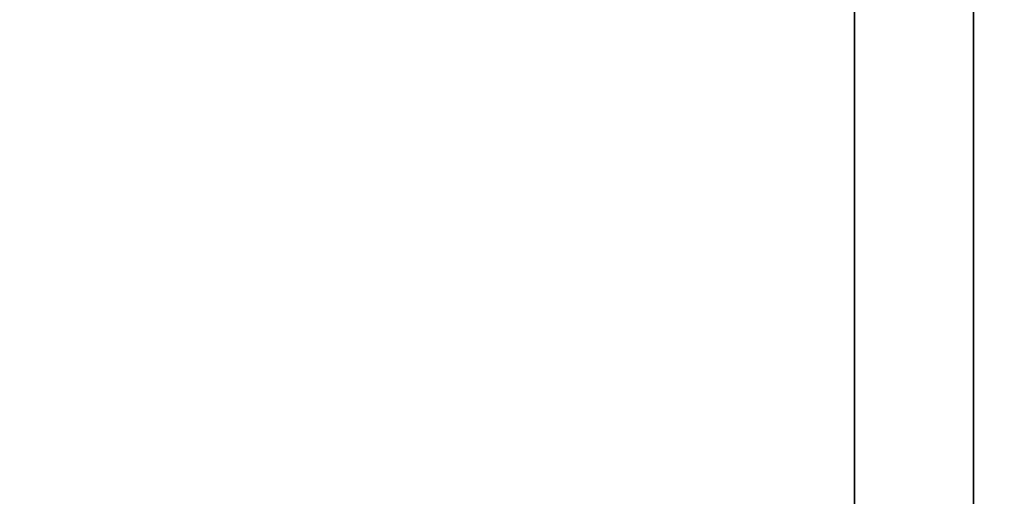
# Model space of a CAD drawing. Units: inches. Extents: x 125 to 976, y 231 to 853.
# Tile 8 of 16: x 393 to 468, y 519 to 555. Entities that reach past the tile are written whole.
import ezdxf

# ---------------------------------------------------------------- set-up
doc = ezdxf.new("R2010")
doc.units = ezdxf.units.IN
doc.header["$MEASUREMENT"] = 0
doc.layers.add('A-ANNO-DIMS', color=2, linetype='Continuous', lineweight=18)
doc.layers.add('A-WALL', color=7, linetype='Continuous', lineweight=35)
doc.styles.get("Standard").update_dxf_attribs({"font": 'italic8.shx'})
doc.dimstyles.get("Standard").update_dxf_attribs({"dimtxt": 8, "dimasz": 0.18, "dimexe": 0.18, "dimexo": 0.0625, "dimgap": 0.09, "dimtad": 0, "dimtih": 1, "dimtoh": 1, "dimdec": 4, "dimzin": 0, "dimdsep": 46, "dimlunit": 3, "dimtxsty": 'Standard', "dimcen": 0.09, "dimclrt": 4, "dimadec": 0, "dimazin": 0, "dimtfac": 1, "dimtdec": 4, "dimtofl": 0, "dimtmove": 0, "dimatfit": 3, "dimfxl": 1, "dimtolj": 1, "dimtzin": 0, "dimarcsym": 0})

# ---------------------------------------------------------------- blocks, each defined once
blk = doc.blocks.new('*D64')
at = {"layer": 'A-ANNO-DIMS', "color": 0, "lineweight": -2, "transparency": 16777216}
for p, q in [((465.642, 658.828), (494.459, 658.828)), ((494.279, 658.648), (494.279, 561.162)), ((494.279, 451.305), (494.279, 548.792)), ((465.642, 451.125), (494.459, 451.125))]:
    blk.add_line(p, q, dxfattribs=at)
at = {"layer": 'A-ANNO-DIMS', "color": 0, "transparency": 16777216}
for points in [[(494.249, 658.648), (494.309, 658.648), (494.279, 658.828)], [(494.249, 451.305), (494.309, 451.305), (494.279, 451.125)]]:
    blk.add_solid(points, dxfattribs=at)
at = {"layer": 'Defpoints', "color": 0, "transparency": 16777216}
for p in [(465.579, 658.828), (494.279, 658.828), (465.579, 451.125)]:
    blk.add_point(p, dxfattribs=at)
at = {"layer": 'A-ANNO-DIMS', "color": 4, "transparency": 16777216, "insert": (494.279, 554.977), "char_height": 8, "attachment_point": 5}
blk.add_mtext('\\A1;17\'-3 1/2"', dxfattribs=at)

msp = doc.modelspace()

# ---------------------------------------------------------------- linework, layer by layer
at = {"layer": 'A-WALL'}
msp.add_line((456.5792, 503.10475), (456.5792, 614.10475), dxfattribs=at)
msp.add_lwpolyline([(177.5792, 272.10475), (465.5792, 272.10475), (465.5792, 812.10475), (177.5792, 812.10475)], close=True, dxfattribs=at)

# ---------------------------------------------------------------- dimensions: what is measured, and where the dimension line sits
at = {"layer": 'A-ANNO-DIMS'}
dim = msp.add_linear_dim(base=(494.2792, 658.82838), p1=(465.5792, 451.12515), p2=(465.5792, 658.82838), angle=90, dimstyle='Standard', override={"dimdec": 1, "dimlfac": 1, "dimrnd": 0, "dimzin": 1, "dimdsep": 46, "dimlunit": 4, "dimfrac": 2}, dxfattribs=at)
dim.commit()
dim.dimension.update_dxf_attribs({"geometry": '*D64', "text_midpoint": (494.2792, 554.97677)})

doc.saveas('drawing.dxf')
